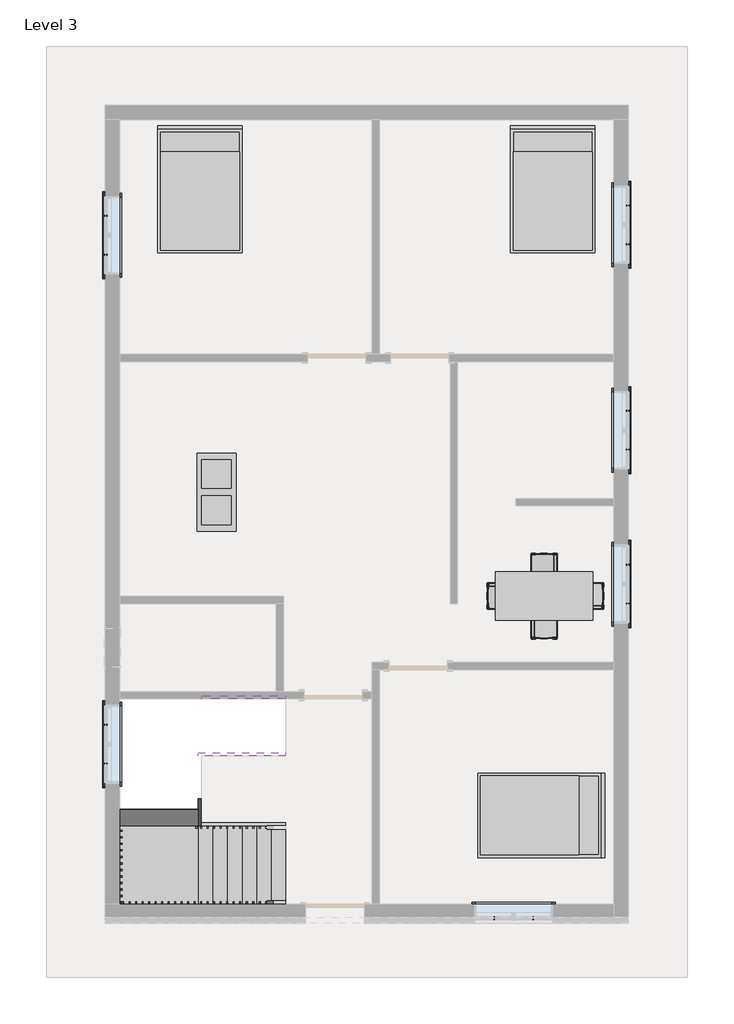
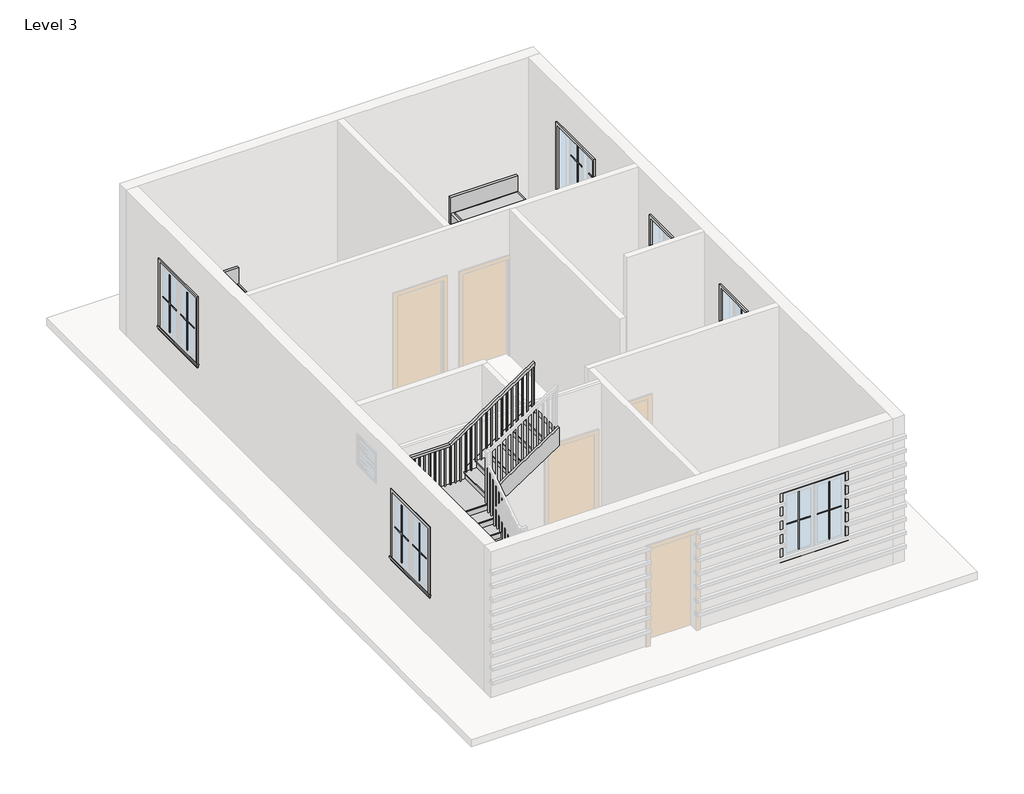
# One storey, part 3 of 3: 25 proxies, 5 members, 4 furniture elements, 1 railing, 1 stair flight.
"""IFC4 building model written with IfcOpenShell, lengths in millimetres."""

from ifc_helpers import new_model, si_unit, frame, origin, place, context, project, spatial, polyline, outline, extrude, faceted_brep, transform, mapped, element, save
from components import muntin_pattern_2x2_muntin_pattern_2x2_ba8901dc, muntin_pattern_2x2_muntin_pattern_2x2_877df4e9, trim_window_exterior_flat_with_sill_fda35bc9, trim_window_interior_flat_picture_frame_a80dbcd9, coffee_table_with_brass_mullions_11320_coffee_table_with_5962bef7, bed_17739_bed_17739_15c61121, dining_table_w_chairs_11374_0cdfc61b, stair_flight_217cdb56

model = new_model("IFC4")

# Units and contexts
model_context = context("Model", 3, world=origin())
ifc_project = project(units=[si_unit("LENGTHUNIT", "METRE", prefix="MILLI")], contexts=[model_context])

# Site, building, storey
site = spatial("IfcSite", under=ifc_project)
building = spatial("IfcBuilding", under=site)
storey = spatial("IfcBuildingStorey", under=building, Name="Level 3", Elevation=6248.4)

# Proxies
placement = place(None, origin())
muntin_pattern_2x2_muntin_pattern_2x2_shape = muntin_pattern_2x2_muntin_pattern_2x2_ba8901dc(model_context)
element("IfcBuildingElementProxy", 1, Name="Muntin Pattern_2x2 : Muntin Pattern_2x2", ObjectType="Muntin Pattern_2x2 : Muntin Pattern_2x2", at=placement, inside=storey, context=model_context, shape_type="MappedRepresentation", body=[
    mapped(muntin_pattern_2x2_muntin_pattern_2x2_shape, transform((-5325.0867403, -4189.9051559, 7232.65), x_axis=(0.0, 1.0, 0.0), y_axis=(-1.0, 0.0, 0.0), z_axis=(0.0, 0.0, 1.0))),
])
element("IfcBuildingElementProxy", 2, Name="Muntin Pattern_2x2 : Muntin Pattern_2x2", ObjectType="Muntin Pattern_2x2 : Muntin Pattern_2x2", at=placement, inside=storey, context=model_context, shape_type="MappedRepresentation", body=[
    mapped(muntin_pattern_2x2_muntin_pattern_2x2_shape, transform((-5325.0867403, 3744.4198441, 7232.65), x_axis=(0.0, 1.0, 0.0), y_axis=(-1.0, 0.0, 0.0), z_axis=(0.0, 0.0, 1.0))),
])
element("IfcBuildingElementProxy", 3, Name="Muntin Pattern_2x2 : Muntin Pattern_2x2", ObjectType="Muntin Pattern_2x2 : Muntin Pattern_2x2", at=placement, inside=storey, context=model_context, shape_type="MappedRepresentation", body=[
    mapped(muntin_pattern_2x2_muntin_pattern_2x2_shape, transform((2821.9632597, 4512.7698441, 7232.65), x_axis=(0.0, -1.0, 0.0), y_axis=(1.0, 0.0, 0.0), z_axis=(0.0, 0.0, 1.0))),
])
element("IfcBuildingElementProxy", 4, Name="Muntin Pattern_2x2 : Muntin Pattern_2x2", ObjectType="Muntin Pattern_2x2 : Muntin Pattern_2x2", at=placement, inside=storey, context=model_context, shape_type="MappedRepresentation", body=[
    mapped(muntin_pattern_2x2_muntin_pattern_2x2_shape, transform((2821.9632597, 1312.3698441, 7232.65), x_axis=(0.0, -1.0, 0.0), y_axis=(1.0, 0.0, 0.0), z_axis=(0.0, 0.0, 1.0))),
])
element("IfcBuildingElementProxy", 5, Name="Muntin Pattern_2x2 : Muntin Pattern_2x2", ObjectType="Muntin Pattern_2x2 : Muntin Pattern_2x2", at=placement, inside=storey, context=model_context, shape_type="MappedRepresentation", body=[
    mapped(muntin_pattern_2x2_muntin_pattern_2x2_shape, transform((2821.9632597, -1087.9301559, 7232.65), x_axis=(0.0, -1.0, 0.0), y_axis=(1.0, 0.0, 0.0), z_axis=(0.0, 0.0, 1.0))),
])
element("IfcBuildingElementProxy", 6, Name="Muntin Pattern_2x2 : Muntin Pattern_2x2", ObjectType="Muntin Pattern_2x2 : Muntin Pattern_2x2", at=placement, inside=storey, context=model_context, shape_type="MappedRepresentation", body=[
    mapped(muntin_pattern_2x2_muntin_pattern_2x2_shape, transform((1344.0007597, -6601.3176559, 7232.65), x_axis=(-1.0, 0.0, 0.0), y_axis=(0.0, -1.0, 0.0), z_axis=(0.0, 0.0, 1.0))),
])
muntin_pattern_2x2_muntin_pattern_2x2_2_shape = muntin_pattern_2x2_muntin_pattern_2x2_877df4e9(model_context)
element("IfcBuildingElementProxy", 7, Name="Muntin Pattern_2x2 : Muntin Pattern_2x2", ObjectType="Muntin Pattern_2x2 : Muntin Pattern_2x2", at=placement, inside=storey, context=model_context, shape_type="MappedRepresentation", body=[
    mapped(muntin_pattern_2x2_muntin_pattern_2x2_2_shape, transform((-5325.0867403, -3583.4801559, 7232.65), x_axis=(0.0, -1.0, 0.0), y_axis=(1.0, 0.0, 0.0), z_axis=(0.0, 0.0, 1.0))),
])
element("IfcBuildingElementProxy", 8, Name="Muntin Pattern_2x2 : Muntin Pattern_2x2", ObjectType="Muntin Pattern_2x2 : Muntin Pattern_2x2", at=placement, inside=storey, context=model_context, shape_type="MappedRepresentation", body=[
    mapped(muntin_pattern_2x2_muntin_pattern_2x2_2_shape, transform((-5325.0867403, 4350.8448441, 7232.65), x_axis=(0.0, -1.0, 0.0), y_axis=(1.0, 0.0, 0.0), z_axis=(0.0, 0.0, 1.0))),
])
element("IfcBuildingElementProxy", 9, Name="Muntin Pattern_2x2 : Muntin Pattern_2x2", ObjectType="Muntin Pattern_2x2 : Muntin Pattern_2x2", at=placement, inside=storey, context=model_context, shape_type="MappedRepresentation", body=[
    mapped(muntin_pattern_2x2_muntin_pattern_2x2_2_shape, transform((2821.9632597, 3906.3448441, 7232.65), x_axis=(0.0, 1.0, 0.0), y_axis=(-1.0, 0.0, 0.0), z_axis=(0.0, 0.0, 1.0))),
])
element("IfcBuildingElementProxy", 10, Name="Muntin Pattern_2x2 : Muntin Pattern_2x2", ObjectType="Muntin Pattern_2x2 : Muntin Pattern_2x2", at=placement, inside=storey, context=model_context, shape_type="MappedRepresentation", body=[
    mapped(muntin_pattern_2x2_muntin_pattern_2x2_2_shape, transform((2821.9632597, 705.9448441, 7232.65), x_axis=(0.0, 1.0, 0.0), y_axis=(-1.0, 0.0, 0.0), z_axis=(0.0, 0.0, 1.0))),
])
element("IfcBuildingElementProxy", 11, Name="Muntin Pattern_2x2 : Muntin Pattern_2x2", ObjectType="Muntin Pattern_2x2 : Muntin Pattern_2x2", at=placement, inside=storey, context=model_context, shape_type="MappedRepresentation", body=[
    mapped(muntin_pattern_2x2_muntin_pattern_2x2_2_shape, transform((2821.9632597, -1694.3551559, 7232.65), x_axis=(0.0, 1.0, 0.0), y_axis=(-1.0, 0.0, 0.0), z_axis=(0.0, 0.0, 1.0))),
])
element("IfcBuildingElementProxy", 12, Name="Muntin Pattern_2x2 : Muntin Pattern_2x2", ObjectType="Muntin Pattern_2x2 : Muntin Pattern_2x2", at=placement, inside=storey, context=model_context, shape_type="MappedRepresentation", body=[
    mapped(muntin_pattern_2x2_muntin_pattern_2x2_2_shape, transform((737.5757597, -6601.3176559, 7232.65), x_axis=(1.0, 0.0, 0.0), y_axis=(0.0, 1.0, 0.0), z_axis=(0.0, 0.0, 1.0))),
])
trim_window_exterior_flat_with_sill_shape = trim_window_exterior_flat_with_sill_fda35bc9(model_context)
element("IfcBuildingElementProxy", 13, Name="Trim-Window-Exterior-Flat : with Sill", ObjectType="Trim-Window-Exterior-Flat : with Sill", at=placement, inside=storey, context=model_context, shape_type="MappedRepresentation", body=[
    mapped(trim_window_exterior_flat_with_sill_shape, transform((-5334.6117403, -3886.6926559, 8509.0), x_axis=(0.0, -1.0, 0.0), y_axis=(0.0, 0.0, 1.0), z_axis=(-1.0, 0.0, 0.0))),
])
element("IfcBuildingElementProxy", 14, Name="Trim-Window-Exterior-Flat : with Sill", ObjectType="Trim-Window-Exterior-Flat : with Sill", at=placement, inside=storey, context=model_context, shape_type="MappedRepresentation", body=[
    mapped(trim_window_exterior_flat_with_sill_shape, transform((-5334.6117403, 4047.6323441, 8509.0), x_axis=(0.0, -1.0, 0.0), y_axis=(0.0, 0.0, 1.0), z_axis=(-1.0, 0.0, 0.0))),
])
element("IfcBuildingElementProxy", 15, Name="Trim-Window-Exterior-Flat : with Sill", ObjectType="Trim-Window-Exterior-Flat : with Sill", at=placement, inside=storey, context=model_context, shape_type="MappedRepresentation", body=[
    mapped(trim_window_exterior_flat_with_sill_shape, transform((2831.4882597, 4209.5573441, 8509.0), x_axis=(0.0, 1.0, 0.0), y_axis=(0.0, 0.0, 1.0), z_axis=(1.0, 0.0, 0.0))),
])
element("IfcBuildingElementProxy", 16, Name="Trim-Window-Exterior-Flat : with Sill", ObjectType="Trim-Window-Exterior-Flat : with Sill", at=placement, inside=storey, context=model_context, shape_type="MappedRepresentation", body=[
    mapped(trim_window_exterior_flat_with_sill_shape, transform((2831.4882597, 1009.1573441, 8509.0), x_axis=(0.0, 1.0, 0.0), y_axis=(0.0, 0.0, 1.0), z_axis=(1.0, 0.0, 0.0))),
])
element("IfcBuildingElementProxy", 17, Name="Trim-Window-Exterior-Flat : with Sill", ObjectType="Trim-Window-Exterior-Flat : with Sill", at=placement, inside=storey, context=model_context, shape_type="MappedRepresentation", body=[
    mapped(trim_window_exterior_flat_with_sill_shape, transform((2831.4882597, -1391.1426559, 8509.0), x_axis=(0.0, 1.0, 0.0), y_axis=(0.0, 0.0, 1.0), z_axis=(1.0, 0.0, 0.0))),
])
element("IfcBuildingElementProxy", 18, Name="Trim-Window-Exterior-Flat : with Sill", ObjectType="Trim-Window-Exterior-Flat : with Sill", at=placement, inside=storey, context=model_context, shape_type="MappedRepresentation", body=[
    mapped(trim_window_exterior_flat_with_sill_shape, transform((1040.7882597, -6610.8426559, 8509.0), x_axis=(1.0, 0.0, 0.0), y_axis=(0.0, 0.0, 1.0), z_axis=(0.0, -1.0, 0.0))),
])
trim_window_interior_flat_picture_frame_shape = trim_window_interior_flat_picture_frame_a80dbcd9(model_context)
element("IfcBuildingElementProxy", 19, Name="Trim-Window-Interior-Flat : Picture Frame", ObjectType="Trim-Window-Interior-Flat : Picture Frame", at=placement, inside=storey, context=model_context, shape_type="MappedRepresentation", body=[
    mapped(trim_window_interior_flat_picture_frame_shape, transform((-5106.0117403, -3886.6926559, 8509.0), x_axis=(0.0, 1.0, 0.0), y_axis=(0.0, 0.0, 1.0), z_axis=(1.0, 0.0, 0.0))),
])
element("IfcBuildingElementProxy", 20, Name="Trim-Window-Interior-Flat : Picture Frame", ObjectType="Trim-Window-Interior-Flat : Picture Frame", at=placement, inside=storey, context=model_context, shape_type="MappedRepresentation", body=[
    mapped(trim_window_interior_flat_picture_frame_shape, transform((-5106.0117403, 4047.6323441, 8509.0), x_axis=(0.0, 1.0, 0.0), y_axis=(0.0, 0.0, 1.0), z_axis=(1.0, 0.0, 0.0))),
])
element("IfcBuildingElementProxy", 21, Name="Trim-Window-Interior-Flat : Picture Frame", ObjectType="Trim-Window-Interior-Flat : Picture Frame", at=placement, inside=storey, context=model_context, shape_type="MappedRepresentation", body=[
    mapped(trim_window_interior_flat_picture_frame_shape, transform((2602.8882597, 4209.5573441, 8509.0), x_axis=(0.0, -1.0, 0.0), y_axis=(0.0, 0.0, 1.0), z_axis=(-1.0, 0.0, 0.0))),
])
element("IfcBuildingElementProxy", 22, Name="Trim-Window-Interior-Flat : Picture Frame", ObjectType="Trim-Window-Interior-Flat : Picture Frame", at=placement, inside=storey, context=model_context, shape_type="MappedRepresentation", body=[
    mapped(trim_window_interior_flat_picture_frame_shape, transform((2602.8882597, 1009.1573441, 8509.0), x_axis=(0.0, -1.0, 0.0), y_axis=(0.0, 0.0, 1.0), z_axis=(-1.0, 0.0, 0.0))),
])
element("IfcBuildingElementProxy", 23, Name="Trim-Window-Interior-Flat : Picture Frame", ObjectType="Trim-Window-Interior-Flat : Picture Frame", at=placement, inside=storey, context=model_context, shape_type="MappedRepresentation", body=[
    mapped(trim_window_interior_flat_picture_frame_shape, transform((2602.8882597, -1391.1426559, 8509.0), x_axis=(0.0, -1.0, 0.0), y_axis=(0.0, 0.0, 1.0), z_axis=(-1.0, 0.0, 0.0))),
])
element("IfcBuildingElementProxy", 24, Name="Trim-Window-Interior-Flat : Picture Frame", ObjectType="Trim-Window-Interior-Flat : Picture Frame", at=placement, inside=storey, context=model_context, shape_type="MappedRepresentation", body=[
    mapped(trim_window_interior_flat_picture_frame_shape, transform((1040.7882597, -6382.2426559, 8509.0), x_axis=(-1.0, 0.0, 0.0), y_axis=(0.0, 0.0, 1.0), z_axis=(0.0, 1.0, 0.0))),
])
coffee_table_with_brass_mullions_11320_coffee_table_with_shape = coffee_table_with_brass_mullions_11320_coffee_table_with_5962bef7(model_context)
element("IfcBuildingElementProxy", 25, Name="coffee_table_with_brass_mullions_11320 : coffee_table_with_brass_mullions_11320", ObjectType="coffee_table_with_brass_mullions_11320 : coffee_table_with_brass_mullions_11320", at=placement, inside=storey, context=model_context, shape_type="MappedRepresentation", body=[
    mapped(coffee_table_with_brass_mullions_11320_coffee_table_with_shape, transform((-3162.9117403, 678.9573441, 6248.4), x_axis=(0.0, 1.0, 0.0), y_axis=(-1.0, 0.0, 0.0), z_axis=(0.0, 0.0, 1.0))),
])

# Furniture
bed_17739_bed_17739_shape = bed_17739_bed_17739_15c61121(model_context)
element("IfcFurniture", 26, ObjectType="Bed_17739 : Bed_17739", at=placement, inside=storey, context=model_context, shape_type="MappedRepresentation", body=[
    mapped(bed_17739_bed_17739_shape, transform((-3855.0617403, 4742.9573441, 6248.4), x_axis=(1.0, 0.0, 0.0), y_axis=(0.0, 1.0, 0.0), z_axis=(0.0, 0.0, 1.0))),
])
element("IfcFurniture", 27, ObjectType="Bed_17739 : Bed_17739", at=placement, inside=storey, context=model_context, shape_type="MappedRepresentation", body=[
    mapped(bed_17739_bed_17739_shape, transform((1650.3882597, 4742.9573441, 6248.4), x_axis=(1.0, 0.0, 0.0), y_axis=(0.0, 1.0, 0.0), z_axis=(0.0, 0.0, 1.0))),
])
element("IfcFurniture", 28, ObjectType="Bed_17739 : Bed_17739", at=placement, inside=storey, context=model_context, shape_type="MappedRepresentation", body=[
    mapped(bed_17739_bed_17739_shape, transform((1447.1882597, -4997.9426559, 6248.4), x_axis=(0.0, -1.0, 0.0), y_axis=(1.0, 0.0, 0.0), z_axis=(0.0, 0.0, 1.0))),
])
dining_table_w_chairs_11374_shape = dining_table_w_chairs_11374_0cdfc61b(model_context)
element("IfcFurniture", 29, ObjectType="Dining_Table_w_Chairs_11374", at=placement, inside=storey, context=model_context, shape_type="MappedRepresentation", body=[
    mapped(dining_table_w_chairs_11374_shape, transform((1497.0410232, -1671.6886654, 6248.4), x_axis=(1.0, 0.0, 0.0), y_axis=(0.0, 1.0, 0.0), z_axis=(0.0, 0.0, 1.0))),
])

# Members
element("IfcMember", 30, ObjectType="Stringer - 2\" Width", at=placement, inside=storey, context=model_context, shape_type="SweptSolid", body=[
    extrude(outline(polyline([(6248.4, -2515.2117403), (6466.4398409, -2515.2117403), (6720.4398409, -2896.2117403), (6720.4398409, -3445.6977546), (6248.4, -2737.6379933), (6248.4, -2515.2117403)])), frame((0.0, -6433.0426559, 0.0), z_axis=(0.0, 1.0, 0.0), x_axis=(0.0, 0.0, 1.0)), (0.0, 0.0, 1.0), 50.8),
])
element("IfcMember", 31, ObjectType="Stringer - 2\" Width", at=placement, inside=storey, context=model_context, shape_type="SweptSolid", body=[
    extrude(outline(polyline([(8487.7158313, -3277.2117403), (8995.7158313, -2515.2117403), (9362.0398409, -2515.2117403), (8487.7158313, -3826.6977546), (8487.7158313, -3277.2117403)])), frame((0.0, -3181.8426559, 0.0), z_axis=(0.0, 1.0, 0.0), x_axis=(0.0, 0.0, 1.0)), (0.0, 0.0, 1.0), 50.8),
])
element("IfcMember", 32, ObjectType="Stringer - 2\" Width", at=placement, inside=storey, context=model_context, shape_type="SweptSolid", body=[
    extrude(outline(polyline([(6248.4, -2515.2117403), (6466.4398409, -2515.2117403), (7346.9731743, -3836.0117403), (6980.6491647, -3836.0117403), (6248.4, -2737.6379933), (6248.4, -2515.2117403)])), frame((0.0, -5163.0426559, 0.0), z_axis=(0.0, 1.0, 0.0), x_axis=(0.0, 0.0, 1.0)), (0.0, 0.0, 1.0), 50.8),
])
element("IfcMember", 33, ObjectType="Stringer - 2\" Width", at=placement, inside=storey, context=model_context, shape_type="SweptSolid", body=[
    extrude(outline(polyline([(-5163.0426559, 7166.9158313), (-5163.0426559, 7533.2398409), (-4070.8426559, 8261.3731743), (-4070.8426559, 7895.0491647), (-5163.0426559, 7166.9158313)])), frame((-3886.8117403, 0.0, 0.0), z_axis=(1.0, 0.0, 0.0), x_axis=(0.0, 1.0, 0.0)), (0.0, 0.0, 1.0), 50.8),
])
element("IfcMember", 34, ObjectType="Stringer - 2\" Width", at=placement, inside=storey, context=model_context, shape_type="SweptSolid", body=[
    extrude(outline(polyline([(8447.6398409, -3886.8117403), (8081.3158313, -3886.8117403), (8995.7158313, -2515.2117403), (9362.0398409, -2515.2117403), (8447.6398409, -3886.8117403)])), frame((0.0, -4070.8426559, 0.0), z_axis=(0.0, 1.0, 0.0), x_axis=(0.0, 0.0, 1.0)), (0.0, 0.0, 1.0), 50.8),
])

# Railing
element("IfcRailing", 35, ObjectType="Handrail - Rectangular", at=placement, inside=storey, context=model_context, shape_type="SolidModel", body=[
    faceted_brep([(-2515.2117403, -6382.2426559, 7315.2), (-2515.2117403, -6382.2426559, 7254.1459984), (-2515.2117403, -6331.4426559, 7254.1459984), (-2515.2117403, -6331.4426559, 7315.2), (-4001.1117403, -6382.2426559, 8305.8), (-4016.4927427, -6382.2426559, 8255.0), (-4016.4927427, -6331.4426559, 8255.0), (-4001.1117403, -6331.4426559, 8305.8), (-5106.0117403, -6382.2426559, 8305.8), (-5106.0117403, -6382.2426559, 8255.0), (-5055.2117403, -6331.4426559, 8255.0), (-5055.2117403, -6331.4426559, 8305.8), (-5106.0117403, -5277.3426559, 8305.8), (-5106.0117403, -5261.9616535, 8255.0), (-5055.2117403, -5261.9616535, 8255.0), (-5055.2117403, -5277.3426559, 8305.8), (-5106.0117403, -4096.2426559, 9093.2), (-5106.0117403, -4080.8616535, 9042.4), (-5055.2117403, -4080.8616535, 9042.4), (-5055.2117403, -4096.2426559, 9093.2), (-5106.0117403, -3181.8426559, 9093.2), (-5106.0117403, -3181.8426559, 9042.4), (-5055.2117403, -3232.6426559, 9042.4), (-5055.2117403, -3232.6426559, 9093.2), (-4191.6117403, -3181.8426559, 9093.2), (-4176.2307379, -3181.8426559, 9042.4), (-4176.2307379, -3232.6426559, 9042.4), (-4191.6117403, -3232.6426559, 9093.2), (-2515.2117403, -3181.8426559, 10210.8), (-2515.2117403, -3232.6426559, 10210.8), (-2515.2117403, -3232.6426559, 10149.7459984), (-2515.2117403, -3181.8426559, 10149.7459984)], [[[0, 1, 2, 3]], [[1, 0, 4, 5]], [[2, 1, 5, 6]], [[3, 2, 6, 7]], [[0, 3, 7, 4]], [[5, 4, 8, 9]], [[6, 5, 9, 10]], [[7, 6, 10, 11]], [[4, 7, 11, 8]], [[9, 8, 12, 13]], [[10, 9, 13, 14]], [[11, 10, 14, 15]], [[8, 11, 15, 12]], [[13, 12, 16, 17]], [[14, 13, 17, 18]], [[15, 14, 18, 19]], [[12, 15, 19, 16]], [[17, 16, 20, 21]], [[18, 17, 21, 22]], [[19, 18, 22, 23]], [[16, 19, 23, 20]], [[21, 20, 24, 25]], [[22, 21, 25, 26]], [[23, 22, 26, 27]], [[20, 23, 27, 24]], [[28, 29, 30, 31]], [[25, 24, 28, 31]], [[26, 25, 31, 30]], [[27, 26, 30, 29]], [[24, 27, 29, 28]]]),
    extrude(outline(polyline([(10126.4626651, -2550.1367403), (9144.0, -2550.1367403), (9144.0, -2531.0867403), (10139.1626651, -2531.0867403), (10126.4626651, -2550.1367403)])), frame((0.0, -3216.7676559, 0.0), z_axis=(0.0, 1.0, 0.0), x_axis=(0.0, 0.0, 1.0)), (0.0, 0.0, 1.0), 19.05),
    extrude(outline(polyline([(10058.7293317, -2651.7367403), (9144.0, -2651.7367403), (9144.0, -2632.6867403), (10071.4293317, -2632.6867403), (10058.7293317, -2651.7367403)])), frame((0.0, -3216.7676559, 0.0), z_axis=(0.0, 1.0, 0.0), x_axis=(0.0, 0.0, 1.0)), (0.0, 0.0, 1.0), 19.05),
    extrude(outline(polyline([(9990.9959984, -2753.3367403), (9144.0, -2753.3367403), (9144.0, -2734.2867403), (10003.6959984, -2734.2867403), (9990.9959984, -2753.3367403)])), frame((0.0, -3216.7676559, 0.0), z_axis=(0.0, 1.0, 0.0), x_axis=(0.0, 0.0, 1.0)), (0.0, 0.0, 1.0), 19.05),
    extrude(outline(polyline([(9923.2626651, -2854.9367403), (8991.6, -2854.9367403), (8991.6, -2835.8867403), (9935.9626651, -2835.8867403), (9923.2626651, -2854.9367403)])), frame((0.0, -3216.7676559, 0.0), z_axis=(0.0, 1.0, 0.0), x_axis=(0.0, 0.0, 1.0)), (0.0, 0.0, 1.0), 19.05),
    extrude(outline(polyline([(9855.5293317, -2956.5367403), (8991.6, -2956.5367403), (8991.6, -2937.4867403), (9868.2293317, -2937.4867403), (9855.5293317, -2956.5367403)])), frame((0.0, -3216.7676559, 0.0), z_axis=(0.0, 1.0, 0.0), x_axis=(0.0, 0.0, 1.0)), (0.0, 0.0, 1.0), 19.05),
    extrude(outline(polyline([(9787.7959984, -3058.1367403), (8839.2, -3058.1367403), (8839.2, -3039.0867403), (9800.4959984, -3039.0867403), (9787.7959984, -3058.1367403)])), frame((0.0, -3216.7676559, 0.0), z_axis=(0.0, 1.0, 0.0), x_axis=(0.0, 0.0, 1.0)), (0.0, 0.0, 1.0), 19.05),
    extrude(outline(polyline([(9720.0626651, -3159.7367403), (8839.2, -3159.7367403), (8839.2, -3140.6867403), (9732.7626651, -3140.6867403), (9720.0626651, -3159.7367403)])), frame((0.0, -3216.7676559, 0.0), z_axis=(0.0, 1.0, 0.0), x_axis=(0.0, 0.0, 1.0)), (0.0, 0.0, 1.0), 19.05),
    extrude(outline(polyline([(9652.3293317, -3261.3367403), (8686.8, -3261.3367403), (8686.8, -3242.2867403), (9665.0293317, -3242.2867403), (9652.3293317, -3261.3367403)])), frame((0.0, -3216.7676559, 0.0), z_axis=(0.0, 1.0, 0.0), x_axis=(0.0, 0.0, 1.0)), (0.0, 0.0, 1.0), 19.05),
    extrude(outline(polyline([(9584.5959984, -3362.9367403), (8686.8, -3362.9367403), (8686.8, -3343.8867403), (9597.2959984, -3343.8867403), (9584.5959984, -3362.9367403)])), frame((0.0, -3216.7676559, 0.0), z_axis=(0.0, 1.0, 0.0), x_axis=(0.0, 0.0, 1.0)), (0.0, 0.0, 1.0), 19.05),
    extrude(outline(polyline([(9516.8626651, -3464.5367403), (8534.4, -3464.5367403), (8534.4, -3445.4867403), (9529.5626651, -3445.4867403), (9516.8626651, -3464.5367403)])), frame((0.0, -3216.7676559, 0.0), z_axis=(0.0, 1.0, 0.0), x_axis=(0.0, 0.0, 1.0)), (0.0, 0.0, 1.0), 19.05),
    extrude(outline(polyline([(9449.1293317, -3566.1367403), (8534.4, -3566.1367403), (8534.4, -3547.0867403), (9461.8293317, -3547.0867403), (9449.1293317, -3566.1367403)])), frame((0.0, -3216.7676559, 0.0), z_axis=(0.0, 1.0, 0.0), x_axis=(0.0, 0.0, 1.0)), (0.0, 0.0, 1.0), 19.05),
    extrude(outline(polyline([(9381.3959984, -3667.7367403), (8534.4, -3667.7367403), (8534.4, -3648.6867403), (9394.0959984, -3648.6867403), (9381.3959984, -3667.7367403)])), frame((0.0, -3216.7676559, 0.0), z_axis=(0.0, 1.0, 0.0), x_axis=(0.0, 0.0, 1.0)), (0.0, 0.0, 1.0), 19.05),
    extrude(outline(polyline([(9313.6626651, -3769.3367403), (8382.0, -3769.3367403), (8382.0, -3750.2867403), (9326.3626651, -3750.2867403), (9313.6626651, -3769.3367403)])), frame((0.0, -3216.7676559, 0.0), z_axis=(0.0, 1.0, 0.0), x_axis=(0.0, 0.0, 1.0)), (0.0, 0.0, 1.0), 19.05),
    extrude(outline(polyline([(9245.9293317, -3870.9367403), (8382.0, -3870.9367403), (8382.0, -3851.8867403), (9258.6293317, -3851.8867403), (9245.9293317, -3870.9367403)])), frame((0.0, -3216.7676559, 0.0), z_axis=(0.0, 1.0, 0.0), x_axis=(0.0, 0.0, 1.0)), (0.0, 0.0, 1.0), 19.05),
    extrude(outline(polyline([(9178.1959984, -3972.5367403), (8229.6, -3972.5367403), (8229.6, -3953.4867403), (9190.8959984, -3953.4867403), (9178.1959984, -3972.5367403)])), frame((0.0, -3216.7676559, 0.0), z_axis=(0.0, 1.0, 0.0), x_axis=(0.0, 0.0, 1.0)), (0.0, 0.0, 1.0), 19.05),
    extrude(outline(polyline([(9110.4626651, -4074.1367403), (8229.6, -4074.1367403), (8229.6, -4055.0867403), (9123.1626651, -4055.0867403), (9110.4626651, -4074.1367403)])), frame((0.0, -3216.7676559, 0.0), z_axis=(0.0, 1.0, 0.0), x_axis=(0.0, 0.0, 1.0)), (0.0, 0.0, 1.0), 19.05),
    extrude(outline(polyline([(9042.7293317, -4175.7367403), (8229.6, -4175.7367403), (8229.6, -4156.6867403), (9055.4293317, -4156.6867403), (9042.7293317, -4175.7367403)])), frame((0.0, -3216.7676559, 0.0), z_axis=(0.0, 1.0, 0.0), x_axis=(0.0, 0.0, 1.0)), (0.0, 0.0, 1.0), 19.05),
    extrude(outline(polyline([(-4277.3367403, -3197.7176559), (-4258.2867403, -3197.7176559), (-4258.2867403, -3216.7676559), (-4277.3367403, -3216.7676559), (-4277.3367403, -3197.7176559)])), frame((0.0, 0.0, 8229.6), z_axis=(0.0, 0.0, 1.0), x_axis=(1.0, 0.0, 0.0)), (0.0, 0.0, 1.0), 812.8),
    extrude(outline(polyline([(-4378.9367403, -3197.7176559), (-4359.8867403, -3197.7176559), (-4359.8867403, -3216.7676559), (-4378.9367403, -3216.7676559), (-4378.9367403, -3197.7176559)])), frame((0.0, 0.0, 8229.6), z_axis=(0.0, 0.0, 1.0), x_axis=(1.0, 0.0, 0.0)), (0.0, 0.0, 1.0), 812.8),
    extrude(outline(polyline([(-4480.5367403, -3197.7176559), (-4461.4867403, -3197.7176559), (-4461.4867403, -3216.7676559), (-4480.5367403, -3216.7676559), (-4480.5367403, -3197.7176559)])), frame((0.0, 0.0, 8229.6), z_axis=(0.0, 0.0, 1.0), x_axis=(1.0, 0.0, 0.0)), (0.0, 0.0, 1.0), 812.8),
    extrude(outline(polyline([(-4582.1367403, -3197.7176559), (-4563.0867403, -3197.7176559), (-4563.0867403, -3216.7676559), (-4582.1367403, -3216.7676559), (-4582.1367403, -3197.7176559)])), frame((0.0, 0.0, 8229.6), z_axis=(0.0, 0.0, 1.0), x_axis=(1.0, 0.0, 0.0)), (0.0, 0.0, 1.0), 812.8),
    extrude(outline(polyline([(-4683.7367403, -3197.7176559), (-4664.6867403, -3197.7176559), (-4664.6867403, -3216.7676559), (-4683.7367403, -3216.7676559), (-4683.7367403, -3197.7176559)])), frame((0.0, 0.0, 8229.6), z_axis=(0.0, 0.0, 1.0), x_axis=(1.0, 0.0, 0.0)), (0.0, 0.0, 1.0), 812.8),
    extrude(outline(polyline([(-4785.3367403, -3197.7176559), (-4766.2867403, -3197.7176559), (-4766.2867403, -3216.7676559), (-4785.3367403, -3216.7676559), (-4785.3367403, -3197.7176559)])), frame((0.0, 0.0, 8229.6), z_axis=(0.0, 0.0, 1.0), x_axis=(1.0, 0.0, 0.0)), (0.0, 0.0, 1.0), 812.8),
    extrude(outline(polyline([(-4886.9367403, -3197.7176559), (-4867.8867403, -3197.7176559), (-4867.8867403, -3216.7676559), (-4886.9367403, -3216.7676559), (-4886.9367403, -3197.7176559)])), frame((0.0, 0.0, 8229.6), z_axis=(0.0, 0.0, 1.0), x_axis=(1.0, 0.0, 0.0)), (0.0, 0.0, 1.0), 812.8),
    extrude(outline(polyline([(-4988.5367403, -3197.7176559), (-4969.4867403, -3197.7176559), (-4969.4867403, -3216.7676559), (-4988.5367403, -3216.7676559), (-4988.5367403, -3197.7176559)])), frame((0.0, 0.0, 8229.6), z_axis=(0.0, 0.0, 1.0), x_axis=(1.0, 0.0, 0.0)), (0.0, 0.0, 1.0), 812.8),
    extrude(outline(polyline([(-5090.1367403, -3318.3676559), (-5090.1367403, -3299.3176559), (-5071.0867403, -3299.3176559), (-5071.0867403, -3318.3676559), (-5090.1367403, -3318.3676559)])), frame((0.0, 0.0, 8229.6), z_axis=(0.0, 0.0, 1.0), x_axis=(1.0, 0.0, 0.0)), (0.0, 0.0, 1.0), 812.8),
    extrude(outline(polyline([(-5090.1367403, -3419.9676559), (-5090.1367403, -3400.9176559), (-5071.0867403, -3400.9176559), (-5071.0867403, -3419.9676559), (-5090.1367403, -3419.9676559)])), frame((0.0, 0.0, 8229.6), z_axis=(0.0, 0.0, 1.0), x_axis=(1.0, 0.0, 0.0)), (0.0, 0.0, 1.0), 812.8),
    extrude(outline(polyline([(-5090.1367403, -3521.5676559), (-5090.1367403, -3502.5176559), (-5071.0867403, -3502.5176559), (-5071.0867403, -3521.5676559), (-5090.1367403, -3521.5676559)])), frame((0.0, 0.0, 8229.6), z_axis=(0.0, 0.0, 1.0), x_axis=(1.0, 0.0, 0.0)), (0.0, 0.0, 1.0), 812.8),
    extrude(outline(polyline([(-5090.1367403, -3623.1676559), (-5090.1367403, -3604.1176559), (-5071.0867403, -3604.1176559), (-5071.0867403, -3623.1676559), (-5090.1367403, -3623.1676559)])), frame((0.0, 0.0, 8229.6), z_axis=(0.0, 0.0, 1.0), x_axis=(1.0, 0.0, 0.0)), (0.0, 0.0, 1.0), 812.8),
    extrude(outline(polyline([(-5090.1367403, -3724.7676559), (-5090.1367403, -3705.7176559), (-5071.0867403, -3705.7176559), (-5071.0867403, -3724.7676559), (-5090.1367403, -3724.7676559)])), frame((0.0, 0.0, 8229.6), z_axis=(0.0, 0.0, 1.0), x_axis=(1.0, 0.0, 0.0)), (0.0, 0.0, 1.0), 812.8),
    extrude(outline(polyline([(-5090.1367403, -3826.3676559), (-5090.1367403, -3807.3176559), (-5071.0867403, -3807.3176559), (-5071.0867403, -3826.3676559), (-5090.1367403, -3826.3676559)])), frame((0.0, 0.0, 8229.6), z_axis=(0.0, 0.0, 1.0), x_axis=(1.0, 0.0, 0.0)), (0.0, 0.0, 1.0), 812.8),
    extrude(outline(polyline([(-5090.1367403, -3927.9676559), (-5090.1367403, -3908.9176559), (-5071.0867403, -3908.9176559), (-5071.0867403, -3927.9676559), (-5090.1367403, -3927.9676559)])), frame((0.0, 0.0, 8229.6), z_axis=(0.0, 0.0, 1.0), x_axis=(1.0, 0.0, 0.0)), (0.0, 0.0, 1.0), 812.8),
    extrude(outline(polyline([(-5090.1367403, -4029.5676559), (-5090.1367403, -4010.5176559), (-5071.0867403, -4010.5176559), (-5071.0867403, -4029.5676559), (-5090.1367403, -4029.5676559)])), frame((0.0, 0.0, 8229.6), z_axis=(0.0, 0.0, 1.0), x_axis=(1.0, 0.0, 0.0)), (0.0, 0.0, 1.0), 812.8),
    extrude(outline(polyline([(-4112.1176559, 9021.5626651), (-4112.1176559, 8077.2), (-4131.1676559, 8077.2), (-4131.1676559, 9008.8626651), (-4112.1176559, 9021.5626651)])), frame((-5090.1367403, 0.0, 0.0), z_axis=(1.0, 0.0, 0.0), x_axis=(0.0, 1.0, 0.0)), (0.0, 0.0, 1.0), 19.05),
    extrude(outline(polyline([(-4213.7176559, 8953.8293317), (-4213.7176559, 8077.2), (-4232.7676559, 8077.2), (-4232.7676559, 8941.1293317), (-4213.7176559, 8953.8293317)])), frame((-5090.1367403, 0.0, 0.0), z_axis=(1.0, 0.0, 0.0), x_axis=(0.0, 1.0, 0.0)), (0.0, 0.0, 1.0), 19.05),
    extrude(outline(polyline([(-4315.3176559, 8886.0959984), (-4315.3176559, 7924.8), (-4334.3676559, 7924.8), (-4334.3676559, 8873.3959984), (-4315.3176559, 8886.0959984)])), frame((-5090.1367403, 0.0, 0.0), z_axis=(1.0, 0.0, 0.0), x_axis=(0.0, 1.0, 0.0)), (0.0, 0.0, 1.0), 19.05),
    extrude(outline(polyline([(-4416.9176559, 8818.3626651), (-4416.9176559, 7924.8), (-4435.9676559, 7924.8), (-4435.9676559, 8805.6626651), (-4416.9176559, 8818.3626651)])), frame((-5090.1367403, 0.0, 0.0), z_axis=(1.0, 0.0, 0.0), x_axis=(0.0, 1.0, 0.0)), (0.0, 0.0, 1.0), 19.05),
    extrude(outline(polyline([(-4518.5176559, 8750.6293317), (-4518.5176559, 7772.4), (-4537.5676559, 7772.4), (-4537.5676559, 8737.9293317), (-4518.5176559, 8750.6293317)])), frame((-5090.1367403, 0.0, 0.0), z_axis=(1.0, 0.0, 0.0), x_axis=(0.0, 1.0, 0.0)), (0.0, 0.0, 1.0), 19.05),
    extrude(outline(polyline([(-4620.1176559, 8682.8959984), (-4620.1176559, 7772.4), (-4639.1676559, 7772.4), (-4639.1676559, 8670.1959984), (-4620.1176559, 8682.8959984)])), frame((-5090.1367403, 0.0, 0.0), z_axis=(1.0, 0.0, 0.0), x_axis=(0.0, 1.0, 0.0)), (0.0, 0.0, 1.0), 19.05),
    extrude(outline(polyline([(-4721.7176559, 8615.1626651), (-4721.7176559, 7620.0), (-4740.7676559, 7620.0), (-4740.7676559, 8602.4626651), (-4721.7176559, 8615.1626651)])), frame((-5090.1367403, 0.0, 0.0), z_axis=(1.0, 0.0, 0.0), x_axis=(0.0, 1.0, 0.0)), (0.0, 0.0, 1.0), 19.05),
    extrude(outline(polyline([(-4823.3176559, 8547.4293317), (-4823.3176559, 7620.0), (-4842.3676559, 7620.0), (-4842.3676559, 8534.7293317), (-4823.3176559, 8547.4293317)])), frame((-5090.1367403, 0.0, 0.0), z_axis=(1.0, 0.0, 0.0), x_axis=(0.0, 1.0, 0.0)), (0.0, 0.0, 1.0), 19.05),
    extrude(outline(polyline([(-4924.9176559, 8479.6959984), (-4924.9176559, 7620.0), (-4943.9676559, 7620.0), (-4943.9676559, 8466.9959984), (-4924.9176559, 8479.6959984)])), frame((-5090.1367403, 0.0, 0.0), z_axis=(1.0, 0.0, 0.0), x_axis=(0.0, 1.0, 0.0)), (0.0, 0.0, 1.0), 19.05),
    extrude(outline(polyline([(-5026.5176559, 8411.9626651), (-5026.5176559, 7467.6), (-5045.5676559, 7467.6), (-5045.5676559, 8399.2626651), (-5026.5176559, 8411.9626651)])), frame((-5090.1367403, 0.0, 0.0), z_axis=(1.0, 0.0, 0.0), x_axis=(0.0, 1.0, 0.0)), (0.0, 0.0, 1.0), 19.05),
    extrude(outline(polyline([(-5128.1176559, 8344.2293317), (-5128.1176559, 7467.6), (-5147.1676559, 7467.6), (-5147.1676559, 8331.5293317), (-5128.1176559, 8344.2293317)])), frame((-5090.1367403, 0.0, 0.0), z_axis=(1.0, 0.0, 0.0), x_axis=(0.0, 1.0, 0.0)), (0.0, 0.0, 1.0), 19.05),
    extrude(outline(polyline([(-5229.7176559, 8276.4959984), (-5229.7176559, 7315.2), (-5248.7676559, 7315.2), (-5248.7676559, 8263.7959984), (-5229.7176559, 8276.4959984)])), frame((-5090.1367403, 0.0, 0.0), z_axis=(1.0, 0.0, 0.0), x_axis=(0.0, 1.0, 0.0)), (0.0, 0.0, 1.0), 19.05),
    extrude(outline(polyline([(-5090.1367403, -5350.3676559), (-5090.1367403, -5331.3176559), (-5071.0867403, -5331.3176559), (-5071.0867403, -5350.3676559), (-5090.1367403, -5350.3676559)])), frame((0.0, 0.0, 7315.2), z_axis=(0.0, 0.0, 1.0), x_axis=(1.0, 0.0, 0.0)), (0.0, 0.0, 1.0), 939.8),
    extrude(outline(polyline([(-5090.1367403, -5451.9676559), (-5090.1367403, -5432.9176559), (-5071.0867403, -5432.9176559), (-5071.0867403, -5451.9676559), (-5090.1367403, -5451.9676559)])), frame((0.0, 0.0, 7315.2), z_axis=(0.0, 0.0, 1.0), x_axis=(1.0, 0.0, 0.0)), (0.0, 0.0, 1.0), 939.8),
    extrude(outline(polyline([(-5090.1367403, -5553.5676559), (-5090.1367403, -5534.5176559), (-5071.0867403, -5534.5176559), (-5071.0867403, -5553.5676559), (-5090.1367403, -5553.5676559)])), frame((0.0, 0.0, 7315.2), z_axis=(0.0, 0.0, 1.0), x_axis=(1.0, 0.0, 0.0)), (0.0, 0.0, 1.0), 939.8),
    extrude(outline(polyline([(-5090.1367403, -5655.1676559), (-5090.1367403, -5636.1176559), (-5071.0867403, -5636.1176559), (-5071.0867403, -5655.1676559), (-5090.1367403, -5655.1676559)])), frame((0.0, 0.0, 7315.2), z_axis=(0.0, 0.0, 1.0), x_axis=(1.0, 0.0, 0.0)), (0.0, 0.0, 1.0), 939.8),
    extrude(outline(polyline([(-5090.1367403, -5756.7676559), (-5090.1367403, -5737.7176559), (-5071.0867403, -5737.7176559), (-5071.0867403, -5756.7676559), (-5090.1367403, -5756.7676559)])), frame((0.0, 0.0, 7315.2), z_axis=(0.0, 0.0, 1.0), x_axis=(1.0, 0.0, 0.0)), (0.0, 0.0, 1.0), 939.8),
    extrude(outline(polyline([(-5090.1367403, -5858.3676559), (-5090.1367403, -5839.3176559), (-5071.0867403, -5839.3176559), (-5071.0867403, -5858.3676559), (-5090.1367403, -5858.3676559)])), frame((0.0, 0.0, 7315.2), z_axis=(0.0, 0.0, 1.0), x_axis=(1.0, 0.0, 0.0)), (0.0, 0.0, 1.0), 939.8),
    extrude(outline(polyline([(-5090.1367403, -5959.9676559), (-5090.1367403, -5940.9176559), (-5071.0867403, -5940.9176559), (-5071.0867403, -5959.9676559), (-5090.1367403, -5959.9676559)])), frame((0.0, 0.0, 7315.2), z_axis=(0.0, 0.0, 1.0), x_axis=(1.0, 0.0, 0.0)), (0.0, 0.0, 1.0), 939.8),
    extrude(outline(polyline([(-5090.1367403, -6061.5676559), (-5090.1367403, -6042.5176559), (-5071.0867403, -6042.5176559), (-5071.0867403, -6061.5676559), (-5090.1367403, -6061.5676559)])), frame((0.0, 0.0, 7315.2), z_axis=(0.0, 0.0, 1.0), x_axis=(1.0, 0.0, 0.0)), (0.0, 0.0, 1.0), 939.8),
    extrude(outline(polyline([(-5090.1367403, -6163.1676559), (-5090.1367403, -6144.1176559), (-5071.0867403, -6144.1176559), (-5071.0867403, -6163.1676559), (-5090.1367403, -6163.1676559)])), frame((0.0, 0.0, 7315.2), z_axis=(0.0, 0.0, 1.0), x_axis=(1.0, 0.0, 0.0)), (0.0, 0.0, 1.0), 939.8),
    extrude(outline(polyline([(-5090.1367403, -6264.7676559), (-5090.1367403, -6245.7176559), (-5071.0867403, -6245.7176559), (-5071.0867403, -6264.7676559), (-5090.1367403, -6264.7676559)])), frame((0.0, 0.0, 7315.2), z_axis=(0.0, 0.0, 1.0), x_axis=(1.0, 0.0, 0.0)), (0.0, 0.0, 1.0), 939.8),
    extrude(outline(polyline([(-5045.6867403, -6366.3676559), (-5064.7367403, -6366.3676559), (-5064.7367403, -6347.3176559), (-5045.6867403, -6347.3176559), (-5045.6867403, -6366.3676559)])), frame((0.0, 0.0, 7315.2), z_axis=(0.0, 0.0, 1.0), x_axis=(1.0, 0.0, 0.0)), (0.0, 0.0, 1.0), 939.8),
    extrude(outline(polyline([(-4944.0867403, -6366.3676559), (-4963.1367403, -6366.3676559), (-4963.1367403, -6347.3176559), (-4944.0867403, -6347.3176559), (-4944.0867403, -6366.3676559)])), frame((0.0, 0.0, 7315.2), z_axis=(0.0, 0.0, 1.0), x_axis=(1.0, 0.0, 0.0)), (0.0, 0.0, 1.0), 939.8),
    extrude(outline(polyline([(-4842.4867403, -6366.3676559), (-4861.5367403, -6366.3676559), (-4861.5367403, -6347.3176559), (-4842.4867403, -6347.3176559), (-4842.4867403, -6366.3676559)])), frame((0.0, 0.0, 7315.2), z_axis=(0.0, 0.0, 1.0), x_axis=(1.0, 0.0, 0.0)), (0.0, 0.0, 1.0), 939.8),
    extrude(outline(polyline([(-4740.8867403, -6366.3676559), (-4759.9367403, -6366.3676559), (-4759.9367403, -6347.3176559), (-4740.8867403, -6347.3176559), (-4740.8867403, -6366.3676559)])), frame((0.0, 0.0, 7315.2), z_axis=(0.0, 0.0, 1.0), x_axis=(1.0, 0.0, 0.0)), (0.0, 0.0, 1.0), 939.8),
    extrude(outline(polyline([(-4639.2867403, -6366.3676559), (-4658.3367403, -6366.3676559), (-4658.3367403, -6347.3176559), (-4639.2867403, -6347.3176559), (-4639.2867403, -6366.3676559)])), frame((0.0, 0.0, 7315.2), z_axis=(0.0, 0.0, 1.0), x_axis=(1.0, 0.0, 0.0)), (0.0, 0.0, 1.0), 939.8),
    extrude(outline(polyline([(-4537.6867403, -6366.3676559), (-4556.7367403, -6366.3676559), (-4556.7367403, -6347.3176559), (-4537.6867403, -6347.3176559), (-4537.6867403, -6366.3676559)])), frame((0.0, 0.0, 7315.2), z_axis=(0.0, 0.0, 1.0), x_axis=(1.0, 0.0, 0.0)), (0.0, 0.0, 1.0), 939.8),
    extrude(outline(polyline([(-4436.0867403, -6366.3676559), (-4455.1367403, -6366.3676559), (-4455.1367403, -6347.3176559), (-4436.0867403, -6347.3176559), (-4436.0867403, -6366.3676559)])), frame((0.0, 0.0, 7315.2), z_axis=(0.0, 0.0, 1.0), x_axis=(1.0, 0.0, 0.0)), (0.0, 0.0, 1.0), 939.8),
    extrude(outline(polyline([(-4334.4867403, -6366.3676559), (-4353.5367403, -6366.3676559), (-4353.5367403, -6347.3176559), (-4334.4867403, -6347.3176559), (-4334.4867403, -6366.3676559)])), frame((0.0, 0.0, 7315.2), z_axis=(0.0, 0.0, 1.0), x_axis=(1.0, 0.0, 0.0)), (0.0, 0.0, 1.0), 939.8),
    extrude(outline(polyline([(-4232.8867403, -6366.3676559), (-4251.9367403, -6366.3676559), (-4251.9367403, -6347.3176559), (-4232.8867403, -6347.3176559), (-4232.8867403, -6366.3676559)])), frame((0.0, 0.0, 7315.2), z_axis=(0.0, 0.0, 1.0), x_axis=(1.0, 0.0, 0.0)), (0.0, 0.0, 1.0), 939.8),
    extrude(outline(polyline([(-4131.2867403, -6366.3676559), (-4150.3367403, -6366.3676559), (-4150.3367403, -6347.3176559), (-4131.2867403, -6347.3176559), (-4131.2867403, -6366.3676559)])), frame((0.0, 0.0, 7315.2), z_axis=(0.0, 0.0, 1.0), x_axis=(1.0, 0.0, 0.0)), (0.0, 0.0, 1.0), 939.8),
    extrude(outline(polyline([(-4029.6867403, -6366.3676559), (-4048.7367403, -6366.3676559), (-4048.7367403, -6347.3176559), (-4029.6867403, -6347.3176559), (-4029.6867403, -6366.3676559)])), frame((0.0, 0.0, 7315.2), z_axis=(0.0, 0.0, 1.0), x_axis=(1.0, 0.0, 0.0)), (0.0, 0.0, 1.0), 939.8),
    extrude(outline(polyline([(8208.7626651, -3947.1367403), (7315.2, -3947.1367403), (7315.2, -3928.0867403), (8196.0626651, -3928.0867403), (8208.7626651, -3947.1367403)])), frame((0.0, -6366.3676559, 0.0), z_axis=(0.0, 1.0, 0.0), x_axis=(0.0, 0.0, 1.0)), (0.0, 0.0, 1.0), 19.05),
    extrude(outline(polyline([(8141.0293317, -3845.5367403), (7162.8, -3845.5367403), (7162.8, -3826.4867403), (8128.3293317, -3826.4867403), (8141.0293317, -3845.5367403)])), frame((0.0, -6366.3676559, 0.0), z_axis=(0.0, 1.0, 0.0), x_axis=(0.0, 0.0, 1.0)), (0.0, 0.0, 1.0), 19.05),
    extrude(outline(polyline([(8073.2959984, -3743.9367403), (7162.8, -3743.9367403), (7162.8, -3724.8867403), (8060.5959984, -3724.8867403), (8073.2959984, -3743.9367403)])), frame((0.0, -6366.3676559, 0.0), z_axis=(0.0, 1.0, 0.0), x_axis=(0.0, 0.0, 1.0)), (0.0, 0.0, 1.0), 19.05),
    extrude(outline(polyline([(8005.5626651, -3642.3367403), (7010.4, -3642.3367403), (7010.4, -3623.2867403), (7992.8626651, -3623.2867403), (8005.5626651, -3642.3367403)])), frame((0.0, -6366.3676559, 0.0), z_axis=(0.0, 1.0, 0.0), x_axis=(0.0, 0.0, 1.0)), (0.0, 0.0, 1.0), 19.05),
    extrude(outline(polyline([(7937.8293317, -3540.7367403), (7010.4, -3540.7367403), (7010.4, -3521.6867403), (7925.1293317, -3521.6867403), (7937.8293317, -3540.7367403)])), frame((0.0, -6366.3676559, 0.0), z_axis=(0.0, 1.0, 0.0), x_axis=(0.0, 0.0, 1.0)), (0.0, 0.0, 1.0), 19.05),
    extrude(outline(polyline([(7870.0959984, -3439.1367403), (7010.4, -3439.1367403), (7010.4, -3420.0867403), (7857.3959984, -3420.0867403), (7870.0959984, -3439.1367403)])), frame((0.0, -6366.3676559, 0.0), z_axis=(0.0, 1.0, 0.0), x_axis=(0.0, 0.0, 1.0)), (0.0, 0.0, 1.0), 19.05),
    extrude(outline(polyline([(7802.3626651, -3337.5367403), (6858.0, -3337.5367403), (6858.0, -3318.4867403), (7789.6626651, -3318.4867403), (7802.3626651, -3337.5367403)])), frame((0.0, -6366.3676559, 0.0), z_axis=(0.0, 1.0, 0.0), x_axis=(0.0, 0.0, 1.0)), (0.0, 0.0, 1.0), 19.05),
    extrude(outline(polyline([(7734.6293317, -3235.9367403), (6858.0, -3235.9367403), (6858.0, -3216.8867403), (7721.9293317, -3216.8867403), (7734.6293317, -3235.9367403)])), frame((0.0, -6366.3676559, 0.0), z_axis=(0.0, 1.0, 0.0), x_axis=(0.0, 0.0, 1.0)), (0.0, 0.0, 1.0), 19.05),
    extrude(outline(polyline([(7666.8959984, -3134.3367403), (6705.6, -3134.3367403), (6705.6, -3115.2867403), (7654.1959984, -3115.2867403), (7666.8959984, -3134.3367403)])), frame((0.0, -6366.3676559, 0.0), z_axis=(0.0, 1.0, 0.0), x_axis=(0.0, 0.0, 1.0)), (0.0, 0.0, 1.0), 19.05),
    extrude(outline(polyline([(7599.1626651, -3032.7367403), (6705.6, -3032.7367403), (6705.6, -3013.6867403), (7586.4626651, -3013.6867403), (7599.1626651, -3032.7367403)])), frame((0.0, -6366.3676559, 0.0), z_axis=(0.0, 1.0, 0.0), x_axis=(0.0, 0.0, 1.0)), (0.0, 0.0, 1.0), 19.05),
    extrude(outline(polyline([(7531.4293317, -2931.1367403), (6553.2, -2931.1367403), (6553.2, -2912.0867403), (7518.7293317, -2912.0867403), (7531.4293317, -2931.1367403)])), frame((0.0, -6366.3676559, 0.0), z_axis=(0.0, 1.0, 0.0), x_axis=(0.0, 0.0, 1.0)), (0.0, 0.0, 1.0), 19.05),
    extrude(outline(polyline([(7463.6959984, -2829.5367403), (6553.2, -2829.5367403), (6553.2, -2810.4867403), (7450.9959984, -2810.4867403), (7463.6959984, -2829.5367403)])), frame((0.0, -6366.3676559, 0.0), z_axis=(0.0, 1.0, 0.0), x_axis=(0.0, 0.0, 1.0)), (0.0, 0.0, 1.0), 19.05),
    extrude(outline(polyline([(7395.9626651, -2727.9367403), (6400.8, -2727.9367403), (6400.8, -2708.8867403), (7383.2626651, -2708.8867403), (7395.9626651, -2727.9367403)])), frame((0.0, -6366.3676559, 0.0), z_axis=(0.0, 1.0, 0.0), x_axis=(0.0, 0.0, 1.0)), (0.0, 0.0, 1.0), 19.05),
    extrude(outline(polyline([(7328.2293317, -2626.3367403), (6400.8, -2626.3367403), (6400.8, -2607.2867403), (7315.5293317, -2607.2867403), (7328.2293317, -2626.3367403)])), frame((0.0, -6366.3676559, 0.0), z_axis=(0.0, 1.0, 0.0), x_axis=(0.0, 0.0, 1.0)), (0.0, 0.0, 1.0), 19.05),
    extrude(outline(polyline([(-5090.1367403, -3216.7676559), (-5090.1367403, -3197.7176559), (-5071.0867403, -3197.7176559), (-5071.0867403, -3216.7676559), (-5090.1367403, -3216.7676559)])), frame((0.0, 0.0, 8229.6), z_axis=(0.0, 0.0, 1.0), x_axis=(1.0, 0.0, 0.0)), (0.0, 0.0, 1.0), 812.8),
    extrude(outline(polyline([(-5071.0867403, -6366.3676559), (-5090.1367403, -6366.3676559), (-5090.1367403, -6347.3176559), (-5071.0867403, -6347.3176559), (-5071.0867403, -6366.3676559)])), frame((0.0, 0.0, 7315.2), z_axis=(0.0, 0.0, 1.0), x_axis=(1.0, 0.0, 0.0)), (0.0, 0.0, 1.0), 939.8),
    extrude(outline(polyline([(10137.0459984, -2534.2617403), (9144.0, -2534.2617403), (9144.0, -2515.2117403), (10149.7459984, -2515.2117403), (10137.0459984, -2534.2617403)])), frame((0.0, -3216.7676559, 0.0), z_axis=(0.0, 1.0, 0.0), x_axis=(0.0, 0.0, 1.0)), (0.0, 0.0, 1.0), 19.05),
    extrude(outline(polyline([(7266.8459984, -2534.2617403), (6400.8, -2534.2617403), (6400.8, -2515.2117403), (7254.1459984, -2515.2117403), (7266.8459984, -2534.2617403)])), frame((0.0, -6366.3676559, 0.0), z_axis=(0.0, 1.0, 0.0), x_axis=(0.0, 0.0, 1.0)), (0.0, 0.0, 1.0), 19.05),
])

# Stair flight
stair_flight_shape = stair_flight_217cdb56(model_context)
element("IfcStairFlight", 36, ObjectType="2\" Tread 1\" Nosing 1/4\" Riser", at=placement, inside=storey, context=model_context, shape_type="MappedRepresentation", body=[
    mapped(stair_flight_shape, transform((0.0, 0.0, 0.0), x_axis=(1.0, 0.0, 0.0), y_axis=(0.0, 1.0, 0.0), z_axis=(0.0, 0.0, 1.0))),
])

save(model, "model.ifc")

# Revit data of these elements
# Type "Muntin Pattern_2x2 : Muntin Pattern_2x2"
#   Width [instance default] = 4' - 0"
#   Thickness = 0' - 0 1/2"
#   Height [instance default] = 4' - 0"
#   Distance = 0' - 0 3/4"
#   Interior Material [instance default] = none
#   Exterior Material [instance default] = none
#   Default Elevation = 0
# Type "Trim-Window-Exterior-Flat : with Sill"
#   Trim Width = 0' - 2 1/4"
#   Trim Thickness_Picture Frame = 0' - 1 1/4"
#   Trim Thickness_with Sill = 0' - 0 3/4"
#   Sill Thickness = 0' - 1 1/4"
#   Opening Width [instance default] = 2' - 0"
#   Opening Height [instance default] = 3' - 0"
#   Default Elevation = 4' - 0"
#   Sill = yes
#   Picture Frame = no
#   Trim Material [instance default] = none
# Type "Trim-Window-Interior-Flat : Picture Frame"
#   Trim Thickness_Picture Frame = 0' - 1 1/4"
#   Trim Width = 0' - 2 1/4"
#   Trim Thickness_with Sill = 0' - 0 3/4"
#   Sill Thickness = 0' - 1 1/4"
#   Opening Width [instance default] = 2' - 0"
#   Opening Height [instance default] = 3' - 0"
#   Default Elevation = 4' - 0"
#   Sill = no
#   Picture Frame = yes
#   Trim Material [instance default] = none
# Type "coffee_table_with_brass_mullions_11320 : coffee_table_with_brass_mullions_11320"
#   Default Elevation = 0
# Type "Bed_17739 : Bed_17739"
#   Default Elevation = 0
# Type "Dining_Table_w_Chairs_11374"
#   Default Elevation = 0
#   Assembly Code = ""
# Type "Handrail - Rectangular"
#   Assembly Code = "C2010400"
#   built-in parameter 1008612 = 0.0416667 (stored number, unit not read)
#   built-in parameter 1008611 = 0.0416667 (stored number, unit not read)
#   built-in parameter 1008609 = 0.333333 (stored number, unit not read)
#   built-in parameter 1008604 = 0.166667 (stored number, unit not read)
#   built-in parameter 1008603 = 0.166667 (stored number, unit not read)
#   Railing Height = 3' - 0"
#   built-in parameter 1008630 = 2
#   built-in parameter 1008610 = 2
#   built-in parameter 1008618 = Baluster - Square : 3/4"
# Elements 1, 2, 3, 4, 5, 6, 7, 8, 9, 10, 11, 12 (IfcBuildingElementProxy, "Muntin Pattern_2x2 : Muntin Pattern_2x2")
#   Width = 1' - 6 5/8"
#   Height = 3' - 11 1/2"
#   Interior Material = Wood - Stained
#   Exterior Material = Clad - White
#   Phase Created = New Construction
#   Materials on its faces: "Clad - White", "Wood - Stained"
# Elements 13, 14, 15, 16, 17, 18 (IfcBuildingElementProxy, "Trim-Window-Exterior-Flat : with Sill")
#   Opening Width = 4' - 0"
#   Opening Height = 4' - 5"
#   Trim Material = Clad - White
#   Phase Created = New Construction
#   Materials on its faces: "Clad - White"
# Elements 19, 20, 21, 22, 23, 24 (IfcBuildingElementProxy, "Trim-Window-Interior-Flat : Picture Frame")
#   Opening Width = 4' - 0"
#   Opening Height = 4' - 5"
#   Trim Material = Wood - Stained
#   Phase Created = New Construction
#   Materials on its faces: "Wood - Stained"
# Element 25 (IfcBuildingElementProxy, "coffee_table_with_brass_mullions_11320 : coffee_table_with_brass_mullions_11320")
#   Phase Created = New Construction
#   Materials on its faces: "Default Wall", "TABLE", "Glass", "Default"
# Elements 26, 27, 28 (IfcFurniture, "Bed_17739 : Bed_17739")
#   Phase Created = New Construction
#   Materials on its faces: "legs", "sheets", "bed frame", "Blanket"
# Element 29 (IfcFurniture, "Dining_Table_w_Chairs_11374")
#   Phase Created = New Construction
# Elements 30, 31, 32, 33, 34 (IfcMember, "Stringer - 2\" Width")
#   Phase Created = New Construction
# Element 35 (IfcRailing, "Handrail - Rectangular")
#   Phase Created = New Construction
#   Materials on its faces: "Clad - White"
# Element 36 (IfcStairFlight, "2\" Tread 1\" Nosing 1/4\" Riser")
#   Phase Created = New Construction
#   Materials on its faces: "Wood Planks"
# Materials
#   "Clad - White": class "Wood", colour RGB 242 242 238, transparency 0, Cost = 0
#   "Wood - Stained": class "Wood", colour RGB 224 178 126, transparency 0, Cost = 0
#   "Default Wall": colour RGB 128 128 128, transparency 0, Cost = 0
#   "TABLE": class "Generic", colour RGB 120 120 120, transparency 0, Cost = 0
#   "Glass": class "Glass", colour RGB 0 128 192, transparency 0.75, Description = "Soda Lime Glass", Cost = 0
#   "Default": colour RGB 127 127 127, transparency 0, Cost = 0
#   "legs": colour RGB 90 73 37, transparency 0, Cost = 0
#   "sheets": colour RGB 200 195 176, transparency 0, Cost = 0
#   "bed frame": colour RGB 90 73 37, transparency 0, Cost = 0
#   "Blanket": class "System", colour RGB 59 0 1, transparency 0, Cost = 0
#   "Wood Planks": class "Wood", colour RGB 193 160 115, transparency 0, Description = "Physical material.", Cost = 0
